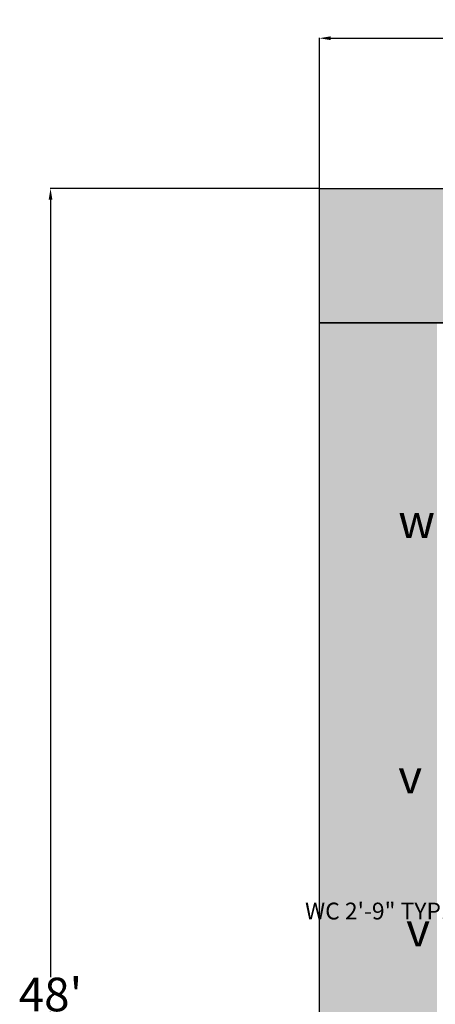
# Model space of a CAD drawing. Units: inches. Extents: x 803 to 1513, y 275 to 951.
# Tile 4 of 10: x 803 to 951, y 599 to 951. Entities that reach past the tile are written whole.
import ezdxf

# ---------------------------------------------------------------- set-up
doc = ezdxf.new("R2010")
doc.units = ezdxf.units.IN
doc.header["$MEASUREMENT"] = 0
for name, color, linetype, lineweight in [('A-ANNO-TEXT', 7, 'Continuous', 18), ('A-WALL', 7, 'Continuous', 35), ('C-PROP', 7, 'Continuous', 25), ('C-SITE-PATT', 9, 'Continuous', 13), ('dim', 1, 'Continuous', 18)]:
    doc.layers.add(name, color=color, linetype=linetype, lineweight=lineweight)
doc.styles.get("Standard").update_dxf_attribs({"font": 'arial.ttf'})
doc.dimstyles.get("Standard").update_dxf_attribs({"dimtxt": 6, "dimasz": 4, "dimexe": 0.18, "dimexo": 0.0625, "dimgap": 0.09, "dimtad": 0, "dimtih": 1, "dimtoh": 1, "dimdec": 0, "dimzin": 0, "dimdsep": 46, "dimlunit": 3, "dimtxsty": 'Standard', "dimcen": 0.09, "dimadec": 0, "dimazin": 0, "dimtfac": 1, "dimtdec": 0, "dimtofl": 0, "dimtmove": 0, "dimatfit": 3, "dimfxl": 1, "dimtolj": 1, "dimtzin": 0, "dimarcsym": 0})

# ---------------------------------------------------------------- blocks, each defined once
blk = doc.blocks.new('*D49')
at = {"layer": 'Defpoints', "color": 0, "transparency": 16777216}
for p in [(1474, 944), (910, 890.25), (1474, 890.25)]:
    blk.add_point(p, dxfattribs=at)
at = {"layer": 'dim', "color": 0, "lineweight": -2, "transparency": 16777216}
for p, q in [((910, 890.31), (910, 944.18)), ((914, 944), (1181.49, 944)), ((1470, 944), (1202.52, 944)), ((1474, 890.31), (1474, 944.18))]:
    blk.add_line(p, q, dxfattribs=at)
at = {"layer": 'dim', "color": 0, "transparency": 16777216}
for points in [[(914, 944.67), (914, 943.33), (910, 944)], [(1470, 944.67), (1470, 943.33), (1474, 944)]]:
    blk.add_solid(points, dxfattribs=at)
at = {"layer": 'dim', "color": 0, "transparency": 16777216, "insert": (1192, 944), "char_height": 6, "attachment_point": 5}
blk.add_mtext("\\A1;{\\H2x;47'}", dxfattribs=at)
blk = doc.blocks.new('*D50')
at = {"layer": 'Defpoints', "color": 0, "transparency": 16777216}
for p in [(910, 890.25), (813.84, 314.25), (910, 314.25)]:
    blk.add_point(p, dxfattribs=at)
at = {"layer": 'dim', "color": 0, "lineweight": -2, "transparency": 16777216}
for p, q in [((909.94, 890.25), (813.66, 890.25)), ((813.84, 886.25), (813.84, 608.47)), ((813.84, 318.25), (813.84, 596.03)), ((909.94, 314.25), (813.66, 314.25))]:
    blk.add_line(p, q, dxfattribs=at)
at = {"layer": 'dim', "color": 0, "transparency": 16777216}
for points in [[(813.17, 886.25), (814.51, 886.25), (813.84, 890.25)], [(813.17, 318.25), (814.51, 318.25), (813.84, 314.25)]]:
    blk.add_solid(points, dxfattribs=at)
at = {"layer": 'dim', "color": 0, "transparency": 16777216, "insert": (813.84, 602.25), "char_height": 6, "attachment_point": 5}
blk.add_mtext("\\A1;{\\H2x;48'}", dxfattribs=at)
blk = doc.blocks.new('*D85')
at = {"layer": 'Defpoints', "color": 0, "transparency": 16777216}
for p in [(960.95, 632.08), (960.95, 627.12), (994, 627.12)]:
    blk.add_point(p, dxfattribs=at)
at = {"layer": 'dim', "color": 0, "lineweight": -2, "transparency": 16777216}
for p, q in [((960.95, 632.08), (956.95, 632.08)), ((960.95, 627.18), (960.95, 632.26)), ((990, 632.08), (964.95, 632.08)), ((994, 627.18), (994, 632.26))]:
    blk.add_line(p, q, dxfattribs=at)
at = {"layer": 'dim', "color": 0, "transparency": 16777216}
for points in [[(964.95, 632.75), (964.95, 631.41), (960.95, 632.08)], [(990, 632.75), (990, 631.41), (994, 632.08)]]:
    blk.add_solid(points, dxfattribs=at)
at = {"layer": 'dim', "color": 0, "transparency": 16777216, "insert": (930.3, 632.08), "char_height": 6, "attachment_point": 5}
blk.add_mtext('\\A1;WC 2\'-9" TYP.', dxfattribs=at)

msp = doc.modelspace()

# ---------------------------------------------------------------- hatches: boundary and pattern name
at = {"layer": 'C-SITE-PATT'}
h = msp.add_hatch(dxfattribs=at)
h.set_pattern_fill('CROSS', color=256, scale=8)
h.paths.add_polyline_path([(952, 890.25), (910, 890.25), (910, 842.25), (952, 842.25)])
h.paths.add_polyline_path([(952, 842.25), (910, 842.25), (910, 362.25), (952, 362.25)])
h.paths.add_polyline_path([(1082.35, 890.25), (952, 890.25), (952, 842.25), (1082.35, 842.25)])
h.paths.add_polyline_path([(1432, 890.25), (1301.5, 890.25), (1301.5, 842.25), (1432, 842.25)])
h.paths.add_polyline_path([(1474, 890.25), (1432, 890.25), (1432, 842.25), (1474, 842.25)])
h.paths.add_polyline_path([(1474, 842.25), (1432, 842.25), (1432, 716.25), (1432, 362.25), (1474, 362.25)])
h.paths.add_polyline_path([(938.78, 396.85), (953.16, 396.85), (953.16, 421.58), (938.78, 421.58)], flags=9)
h.paths.add_polyline_path([(937.82, 612.92), (952.2, 612.92), (952.2, 637.65), (937.82, 637.65)], flags=9)
h.paths.add_polyline_path([(934.99, 667.62), (949.37, 667.62), (949.37, 692.35), (934.99, 692.35)], flags=24)
h.paths.add_polyline_path([(937.65, 500.72), (955.76, 500.72), (955.76, 525.45), (937.65, 525.45)], flags=9)
h.paths.add_polyline_path([(935.15, 758.83), (953.26, 758.83), (953.26, 783.56), (935.15, 783.56)], flags=9)
h.paths.add_polyline_path([(1011, 836.25), (1029.11, 836.25), (1029.11, 860.97), (1011, 860.97)], flags=9)
h.paths.add_polyline_path([(1346.52, 836.25), (1364.63, 836.25), (1364.63, 860.97), (1346.52, 860.97)], flags=9)
h.paths.add_polyline_path([(1430.4, 388.1), (1444.78, 388.1), (1444.78, 412.82), (1430.4, 412.82)], flags=9)
h.paths.add_polyline_path([(1429.9, 612.17), (1444.28, 612.17), (1444.28, 636.89), (1429.9, 636.89)], flags=9)
h.paths.add_polyline_path([(1429.47, 667.86), (1443.85, 667.86), (1443.85, 692.59), (1429.47, 692.59)], flags=9)
h.paths.add_polyline_path([(1431.88, 500.79), (1449.99, 500.79), (1449.99, 525.52), (1431.88, 525.52)], flags=9)
h.paths.add_polyline_path([(1429.97, 762.25), (1448.08, 762.25), (1448.08, 786.98), (1429.97, 786.98)], flags=9)

# ---------------------------------------------------------------- linework, layer by layer
at = {"layer": 'A-WALL'}
msp.add_line((910, 842.25), (1097, 842.25), dxfattribs=at)
at = {"layer": 'C-PROP'}
for p, q in [((910, 314.25), (910, 890.25)), ((910, 890.25), (1474, 890.25))]:
    msp.add_line(p, q, dxfattribs=at)

# ---------------------------------------------------------------- texts
at = {"layer": 'A-ANNO-TEXT', "char_height": 12, "attachment_point": 1}
for s, insert in [('w', (938.2, 777.39)), ('v', (938.2, 686.17)), ('v', (941.03, 631.48))]:
    msp.add_mtext_dynamic_manual_height_columns(s, width=13.8024, gutter_width=1, heights=[0], dxfattribs=dict(at, insert=insert))

# ---------------------------------------------------------------- dimensions: what is measured, and where the dimension line sits
at = {"layer": 'dim'}
dim = msp.add_linear_dim(base=(1474, 944), p1=(910, 890.25), p2=(1474, 890.25), text='{\\H2x;<>}', dimstyle='Standard', override={"dimclrd": 0, "dimclre": 0, "dimclrt": 0}, dxfattribs=at)
dim.commit()
dim.dimension.update_dxf_attribs({"geometry": '*D49', "text_midpoint": (1192, 944)})
for base, p1, p2, angle, text, override, picture, middle in [((813.84, 314.25), (910, 890.25), (910, 314.25), 90, '{\\H2x;<>}', {"dimclrd": 0, "dimclre": 0, "dimclrt": 0}, '*D50', (813.84, 602.25)), ((960.9496, 632.079), (993.9959, 627.1221), (960.9496, 627.1221), 180, 'WC <> TYP.', {"dimdec": 1, "dimlfac": 1, "dimrnd": 0, "dimzin": 1, "dimdsep": 46, "dimlunit": 4, "dimfrac": 2}, '*D85', (930.3037, 632.079))]:
    dim = msp.add_linear_dim(base=base, p1=p1, p2=p2, angle=angle, text=text, dimstyle='Standard', override=override, dxfattribs=at)
    dim.commit()
    dim.dimension.update_dxf_attribs({"geometry": picture, "text_midpoint": middle})

doc.saveas('drawing.dxf')
